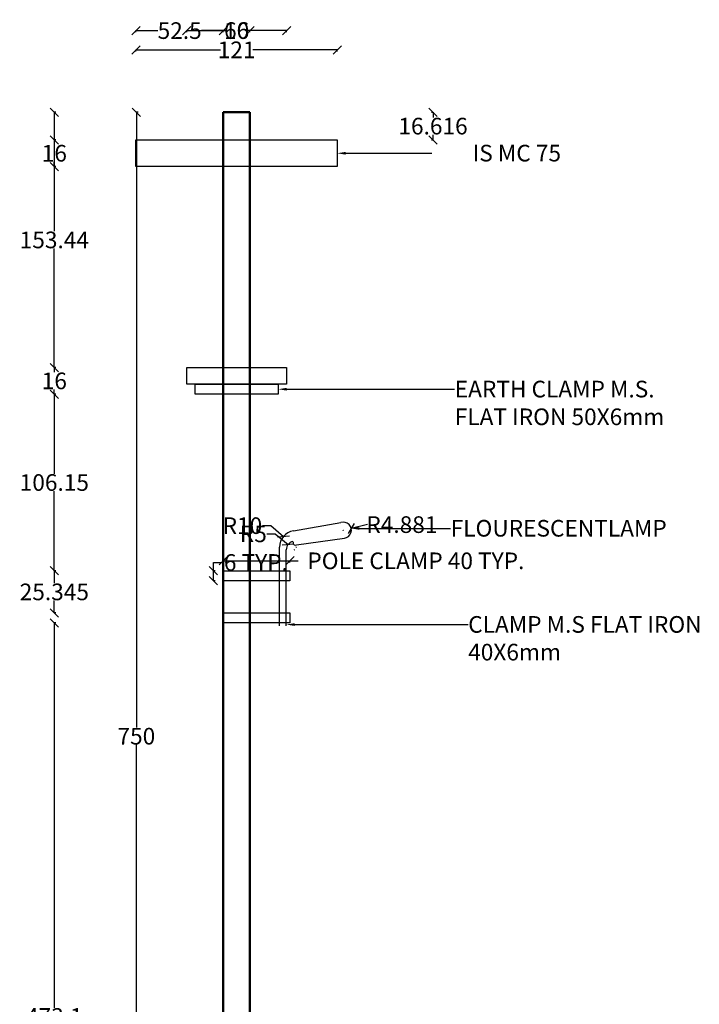
# Model space of a CAD drawing. Units: centimetres. Extents: x -70 to 1009, y -133 to 977.
# Tile 2 of 3: x -70 to 338, y 385 to 977. Entities that reach past the tile are written whole.
import ezdxf
from ezdxf import colors
from ezdxf.entities.mleader import LeaderData, LeaderLine
from ezdxf.math import Vec2, Vec3

# ---------------------------------------------------------------- set-up
doc = ezdxf.new("R2010")
doc.units = ezdxf.units.CM
doc.header["$MEASUREMENT"] = 0
for name, color, linetype, lineweight in [('E-ANNO-DIMS', 2, 'Continuous', 18), ('E-ANNO-TEXT', 7, 'Continuous', 25), ('E-LITE', 3, 'Continuous', 25), ('E-POLE', 7, 'Continuous', 50), ('E-POLE-HDWR', 4, 'Continuous', 25)]:
    doc.layers.add(name, color=color, linetype=linetype, lineweight=lineweight)
doc.styles.get("Standard").update_dxf_attribs({"font": 'arial.ttf'})
doc.dimstyles.get("Standard").update_dxf_attribs({"dimtxt": 10, "dimasz": 5, "dimexe": 0.1, "dimexo": 0.1, "dimgap": 0.09, "dimtad": 0, "dimtih": 1, "dimtoh": 1, "dimdec": 0, "dimzin": 0, "dimdsep": 46, "dimtxsty": 'Standard', "dimblk": 'OBLIQUE', "dimcen": 0.09, "dimadec": 0, "dimazin": 0, "dimtfac": 1, "dimtdec": 0, "dimtofl": 0, "dimtmove": 0, "dimatfit": 3, "dimfxl": 1, "dimfxlon": 1, "dimtolj": 1, "dimtzin": 0, "dimarcsym": 0})

# ---------------------------------------------------------------- blocks, each defined once
blk = doc.blocks.new('_Oblique')
at = {"color": 0, "linetype": 'ByBlock', "lineweight": -2}
blk.add_line((-0.5, -0.5), (0.5, 0.5), dxfattribs=at)
blk = doc.blocks.new('*D1')
at = {"layer": 'Defpoints', "color": 0, "transparency": 16777216}
for p in [(120.74, 958.75), (-0.26, 904.6), (120.74, 904.6)]:
    blk.add_point(p, dxfattribs=at)
at = {"layer": 'E-ANNO-DIMS', "color": 0, "lineweight": -2, "transparency": 16777216}
for p, q in [((-0.26, 957.75), (-0.26, 958.85)), ((-0.26, 958.75), (50.54, 958.75)), ((120.74, 958.75), (69.94, 958.75)), ((120.74, 957.75), (120.74, 958.85))]:
    blk.add_line(p, q, dxfattribs=at)
at = {"layer": 'E-ANNO-DIMS', "color": 0, "lineweight": -2, "transparency": 16777216, "xscale": 5, "yscale": 5, "zscale": 5, "rotation": 180}
blk.add_blockref('_Oblique', (-0.26, 958.75), dxfattribs=at)
at = {"layer": 'E-ANNO-DIMS', "color": 0, "lineweight": -2, "transparency": 16777216, "xscale": 5, "yscale": 5, "zscale": 5}
blk.add_blockref('_Oblique', (120.74, 958.75), dxfattribs=at)
at = {"layer": 'E-ANNO-DIMS', "color": 0, "transparency": 16777216, "insert": (60.24, 958.75), "char_height": 10, "attachment_point": 5}
blk.add_mtext('\\A1;121', dxfattribs=at)
blk = doc.blocks.new('*D3')
at = {"layer": 'Defpoints', "color": 0, "transparency": 16777216}
for p in [(52.24, 921.22), (-0.04, 171.22), (52.24, 171.22)]:
    blk.add_point(p, dxfattribs=at)
at = {"layer": 'E-ANNO-DIMS', "color": 0, "lineweight": -2, "transparency": 16777216}
for p, q in [((0.96, 921.22), (-0.14, 921.22)), ((-0.04, 921.22), (-0.04, 551.41)), ((-0.04, 171.22), (-0.04, 541.02)), ((0.96, 171.22), (-0.14, 171.22))]:
    blk.add_line(p, q, dxfattribs=at)
at = {"layer": 'E-ANNO-DIMS', "color": 0, "lineweight": -2, "transparency": 16777216, "xscale": 5, "yscale": 5, "zscale": 5}
for p, rotation in [((-0.04, 921.22), 90), ((-0.04, 171.22), 270)]:
    blk.add_blockref('_Oblique', p, dxfattribs=dict(at, rotation=rotation))
at = {"layer": 'E-ANNO-DIMS', "color": 0, "transparency": 16777216, "insert": (-0.04, 546.22), "char_height": 10, "attachment_point": 5}
blk.add_mtext('\\A1;750', dxfattribs=at)
blk = doc.blocks.new('POLE-CLAMP')
for p, q in [((0, 0), (0, 6)), ((0, 6), (40, 6)), ((40, 6), (40, 0)), ((40, 0), (0, 0))]:
    blk.add_line(p, q)
blk = doc.blocks.new('*D19')
at = {"layer": 'Defpoints', "color": 0, "transparency": 16777216}
for p in [(92.24, 651.63), (52.24, 645.63), (92.24, 645.63)]:
    blk.add_point(p, dxfattribs=at)
at = {"layer": 'E-ANNO-DIMS', "color": 0, "lineweight": -2, "transparency": 16777216}
for p, q in [((52.24, 650.63), (52.24, 651.73)), ((52.24, 651.63), (92.24, 651.63)), ((92.24, 650.63), (92.24, 651.73)), ((92.24, 651.63), (97.24, 651.63))]:
    blk.add_line(p, q, dxfattribs=at)
at = {"layer": 'E-ANNO-DIMS', "color": 0, "lineweight": -2, "transparency": 16777216, "xscale": 5, "yscale": 5, "zscale": 5, "rotation": 180}
blk.add_blockref('_Oblique', (52.24, 651.63), dxfattribs=at)
at = {"layer": 'E-ANNO-DIMS', "color": 0, "lineweight": -2, "transparency": 16777216, "xscale": 5, "yscale": 5, "zscale": 5}
blk.add_blockref('_Oblique', (92.24, 651.63), dxfattribs=at)
at = {"layer": 'E-ANNO-DIMS', "color": 0, "transparency": 16777216, "insert": (168, 651.63), "char_height": 10, "attachment_point": 5}
blk.add_mtext('\\A1;POLE CLAMP 40 TYP.', dxfattribs=at)
blk = doc.blocks.new('*D20')
at = {"layer": 'Defpoints', "color": 0, "transparency": 16777216}
for p in [(46.24, 645.63), (52.24, 645.63), (52.24, 639.63)]:
    blk.add_point(p, dxfattribs=at)
at = {"layer": 'E-ANNO-DIMS', "color": 0, "lineweight": -2, "transparency": 16777216}
for p, q in [((47.24, 645.63), (46.14, 645.63)), ((46.24, 645.63), (46.24, 650.63)), ((46.24, 650.63), (51.24, 650.63)), ((46.24, 639.63), (46.24, 645.63)), ((47.24, 639.63), (46.14, 639.63))]:
    blk.add_line(p, q, dxfattribs=at)
at = {"layer": 'E-ANNO-DIMS', "color": 0, "lineweight": -2, "transparency": 16777216, "xscale": 5, "yscale": 5, "zscale": 5}
for p, rotation in [((46.24, 645.63), 90), ((46.24, 639.63), 270)]:
    blk.add_blockref('_Oblique', p, dxfattribs=dict(at, rotation=rotation))
at = {"layer": 'E-ANNO-DIMS', "color": 0, "transparency": 16777216, "insert": (71.81, 650.63), "char_height": 10, "attachment_point": 5}
blk.add_mtext('\\A1;6 TYP.', dxfattribs=at)
blk = doc.blocks.new('*D24')
at = {"layer": 'Defpoints', "color": 0, "transparency": 16777216}
for p in [(68.24, 970.32), (52.24, 921.22), (68.24, 921.22)]:
    blk.add_point(p, dxfattribs=at)
at = {"layer": 'E-ANNO-DIMS', "color": 0, "lineweight": -2, "transparency": 16777216}
for p, q in [((52.24, 969.32), (52.24, 970.42)), ((52.24, 970.32), (53.46, 970.32)), ((68.24, 970.32), (67.02, 970.32)), ((68.24, 969.32), (68.24, 970.42))]:
    blk.add_line(p, q, dxfattribs=at)
at = {"layer": 'E-ANNO-DIMS', "color": 0, "lineweight": -2, "transparency": 16777216, "xscale": 5, "yscale": 5, "zscale": 5, "rotation": 180}
blk.add_blockref('_Oblique', (52.24, 970.32), dxfattribs=at)
at = {"layer": 'E-ANNO-DIMS', "color": 0, "lineweight": -2, "transparency": 16777216, "xscale": 5, "yscale": 5, "zscale": 5}
blk.add_blockref('_Oblique', (68.24, 970.32), dxfattribs=at)
at = {"layer": 'E-ANNO-DIMS', "color": 0, "transparency": 16777216, "insert": (60.24, 970.32), "char_height": 10, "attachment_point": 5}
blk.add_mtext('\\A1;16', dxfattribs=at)
blk = doc.blocks.new('*D26')
at = {"layer": 'Defpoints', "color": 0, "transparency": 16777216}
for p in [(68.24, 921.22), (120.74, 904.6), (178.32, 904.6)]:
    blk.add_point(p, dxfattribs=at)
at = {"layer": 'E-ANNO-DIMS', "color": 0, "lineweight": -2, "transparency": 16777216}
for p, q in [((177.32, 921.22), (178.42, 921.22)), ((178.32, 921.22), (178.32, 918.1)), ((178.32, 904.6), (178.32, 907.71)), ((177.32, 904.6), (178.42, 904.6))]:
    blk.add_line(p, q, dxfattribs=at)
at = {"layer": 'E-ANNO-DIMS', "color": 0, "lineweight": -2, "transparency": 16777216, "xscale": 5, "yscale": 5, "zscale": 5}
for p, rotation in [((178.32, 921.22), 90), ((178.32, 904.6), 270)]:
    blk.add_blockref('_Oblique', p, dxfattribs=dict(at, rotation=rotation))
at = {"layer": 'E-ANNO-DIMS', "color": 0, "transparency": 16777216, "insert": (178.32, 912.91), "char_height": 10, "attachment_point": 5}
blk.add_mtext('\\A1;16.616', dxfattribs=at)
blk = doc.blocks.new('*D27')
at = {"layer": 'Defpoints', "color": 0, "transparency": 16777216}
for p in [(-49.36, 904.6), (-0.26, 904.6), (-0.26, 888.6)]:
    blk.add_point(p, dxfattribs=at)
at = {"layer": 'E-ANNO-DIMS', "color": 0, "lineweight": -2, "transparency": 16777216}
for p, q in [((-48.36, 904.6), (-49.46, 904.6)), ((-49.36, 904.6), (-49.36, 901.8)), ((-48.36, 888.6), (-49.46, 888.6)), ((-49.36, 888.6), (-49.36, 891.4))]:
    blk.add_line(p, q, dxfattribs=at)
at = {"layer": 'E-ANNO-DIMS', "color": 0, "lineweight": -2, "transparency": 16777216, "xscale": 5, "yscale": 5, "zscale": 5}
for p, rotation in [((-49.36, 904.6), 90), ((-49.36, 888.6), 270)]:
    blk.add_blockref('_Oblique', p, dxfattribs=dict(at, rotation=rotation))
at = {"layer": 'E-ANNO-DIMS', "color": 0, "transparency": 16777216, "insert": (-49.36, 896.6), "char_height": 10, "attachment_point": 5}
blk.add_mtext('\\A1;16', dxfattribs=at)
blk = doc.blocks.new('*D28')
at = {"layer": 'Defpoints', "color": 0, "transparency": 16777216}
for p in [(52.24, 970.32), (52.24, 921.22), (-0.26, 904.6)]:
    blk.add_point(p, dxfattribs=at)
at = {"layer": 'E-ANNO-DIMS', "color": 0, "lineweight": -2, "transparency": 16777216}
for p, q in [((-0.26, 969.32), (-0.26, 970.42)), ((-0.26, 970.32), (12.87, 970.32)), ((52.24, 970.32), (39.1, 970.32)), ((52.24, 969.32), (52.24, 970.42))]:
    blk.add_line(p, q, dxfattribs=at)
at = {"layer": 'E-ANNO-DIMS', "color": 0, "lineweight": -2, "transparency": 16777216, "xscale": 5, "yscale": 5, "zscale": 5, "rotation": 180}
blk.add_blockref('_Oblique', (-0.26, 970.32), dxfattribs=at)
at = {"layer": 'E-ANNO-DIMS', "color": 0, "lineweight": -2, "transparency": 16777216, "xscale": 5, "yscale": 5, "zscale": 5}
blk.add_blockref('_Oblique', (52.24, 970.32), dxfattribs=at)
at = {"layer": 'E-ANNO-DIMS', "color": 0, "transparency": 16777216, "insert": (25.99, 970.32), "char_height": 10, "attachment_point": 5}
blk.add_mtext('\\A1;52.5', dxfattribs=at)
blk = doc.blocks.new('*D29')
at = {"layer": 'Defpoints', "color": 0, "transparency": 16777216}
for p in [(90.24, 970.32), (30.24, 767.78), (90.24, 767.78)]:
    blk.add_point(p, dxfattribs=at)
at = {"layer": 'E-ANNO-DIMS', "color": 0, "lineweight": -2, "transparency": 16777216}
for p, q in [((30.24, 969.32), (30.24, 970.42)), ((30.24, 970.32), (52.98, 970.32)), ((90.24, 970.32), (67.5, 970.32)), ((90.24, 969.32), (90.24, 970.42))]:
    blk.add_line(p, q, dxfattribs=at)
at = {"layer": 'E-ANNO-DIMS', "color": 0, "lineweight": -2, "transparency": 16777216, "xscale": 5, "yscale": 5, "zscale": 5, "rotation": 180}
blk.add_blockref('_Oblique', (30.24, 970.32), dxfattribs=at)
at = {"layer": 'E-ANNO-DIMS', "color": 0, "lineweight": -2, "transparency": 16777216, "xscale": 5, "yscale": 5, "zscale": 5}
blk.add_blockref('_Oblique', (90.24, 970.32), dxfattribs=at)
at = {"layer": 'E-ANNO-DIMS', "color": 0, "transparency": 16777216, "insert": (60.24, 970.32), "char_height": 10, "attachment_point": 5}
blk.add_mtext('\\A1;60', dxfattribs=at)
blk = doc.blocks.new('*D30')
at = {"layer": 'Defpoints', "color": 0, "transparency": 16777216}
for p in [(30.24, 767.78), (-49.36, 751.78), (35.24, 751.78)]:
    blk.add_point(p, dxfattribs=at)
at = {"layer": 'E-ANNO-DIMS', "color": 0, "lineweight": -2, "transparency": 16777216}
for p, q in [((-48.36, 767.78), (-49.46, 767.78)), ((-49.36, 767.78), (-49.36, 764.97)), ((-48.36, 751.78), (-49.46, 751.78)), ((-49.36, 751.78), (-49.36, 754.58))]:
    blk.add_line(p, q, dxfattribs=at)
at = {"layer": 'E-ANNO-DIMS', "color": 0, "lineweight": -2, "transparency": 16777216, "xscale": 5, "yscale": 5, "zscale": 5}
for p, rotation in [((-49.36, 767.78), 90), ((-49.36, 751.78), 270)]:
    blk.add_blockref('_Oblique', p, dxfattribs=dict(at, rotation=rotation))
at = {"layer": 'E-ANNO-DIMS', "color": 0, "transparency": 16777216, "insert": (-49.36, 759.78), "char_height": 10, "attachment_point": 5}
blk.add_mtext('\\A1;16', dxfattribs=at)
blk = doc.blocks.new('*D31')
at = {"layer": 'Defpoints', "color": 0, "transparency": 16777216}
for p in [(52.24, 921.22), (-49.36, 767.78), (30.24, 767.78)]:
    blk.add_point(p, dxfattribs=at)
at = {"layer": 'E-ANNO-DIMS', "color": 0, "lineweight": -2, "transparency": 16777216}
for p, q in [((-48.36, 921.22), (-49.46, 921.22)), ((-49.36, 921.22), (-49.36, 849.69)), ((-49.36, 767.78), (-49.36, 839.3)), ((-48.36, 767.78), (-49.46, 767.78))]:
    blk.add_line(p, q, dxfattribs=at)
at = {"layer": 'E-ANNO-DIMS', "color": 0, "lineweight": -2, "transparency": 16777216, "xscale": 5, "yscale": 5, "zscale": 5}
for p, rotation in [((-49.36, 921.22), 90), ((-49.36, 767.78), 270)]:
    blk.add_blockref('_Oblique', p, dxfattribs=dict(at, rotation=rotation))
at = {"layer": 'E-ANNO-DIMS', "color": 0, "transparency": 16777216, "insert": (-49.36, 844.5), "char_height": 10, "attachment_point": 5}
blk.add_mtext('\\A1;153.44', dxfattribs=at)
blk = doc.blocks.new('*D32')
at = {"layer": 'Defpoints', "color": 0, "transparency": 16777216}
for p in [(35.24, 751.78), (-49.36, 645.63), (52.24, 645.63)]:
    blk.add_point(p, dxfattribs=at)
at = {"layer": 'E-ANNO-DIMS', "color": 0, "lineweight": -2, "transparency": 16777216}
for p, q in [((-48.36, 751.78), (-49.46, 751.78)), ((-49.36, 751.78), (-49.36, 703.9)), ((-49.36, 645.63), (-49.36, 693.5)), ((-48.36, 645.63), (-49.46, 645.63))]:
    blk.add_line(p, q, dxfattribs=at)
at = {"layer": 'E-ANNO-DIMS', "color": 0, "lineweight": -2, "transparency": 16777216, "xscale": 5, "yscale": 5, "zscale": 5}
for p, rotation in [((-49.36, 751.78), 90), ((-49.36, 645.63), 270)]:
    blk.add_blockref('_Oblique', p, dxfattribs=dict(at, rotation=rotation))
at = {"layer": 'E-ANNO-DIMS', "color": 0, "transparency": 16777216, "insert": (-49.36, 698.7), "char_height": 10, "attachment_point": 5}
blk.add_mtext('\\A1;106.15', dxfattribs=at)
blk = doc.blocks.new('*D33')
at = {"layer": 'Defpoints', "color": 0, "transparency": 16777216}
for p in [(52.24, 645.63), (-49.36, 620.28), (52.24, 620.28)]:
    blk.add_point(p, dxfattribs=at)
at = {"layer": 'E-ANNO-DIMS', "color": 0, "lineweight": -2, "transparency": 16777216}
for p, q in [((-48.36, 645.63), (-49.46, 645.63)), ((-49.36, 645.63), (-49.36, 638.15)), ((-49.36, 620.28), (-49.36, 627.75)), ((-48.36, 620.28), (-49.46, 620.28))]:
    blk.add_line(p, q, dxfattribs=at)
at = {"layer": 'E-ANNO-DIMS', "color": 0, "lineweight": -2, "transparency": 16777216, "xscale": 5, "yscale": 5, "zscale": 5}
for p, rotation in [((-49.36, 645.63), 90), ((-49.36, 620.28), 270)]:
    blk.add_blockref('_Oblique', p, dxfattribs=dict(at, rotation=rotation))
at = {"layer": 'E-ANNO-DIMS', "color": 0, "transparency": 16777216, "insert": (-49.36, 632.95), "char_height": 10, "attachment_point": 5}
blk.add_mtext('\\A1;25.345', dxfattribs=at)
blk = doc.blocks.new('*D34')
at = {"layer": 'Defpoints', "color": 0, "transparency": 16777216}
for p in [(52.24, 614.28), (-49.36, 141.22), (2.39, 141.22)]:
    blk.add_point(p, dxfattribs=at)
at = {"layer": 'E-ANNO-DIMS', "color": 0, "lineweight": -2, "transparency": 16777216}
for p, q in [((-48.36, 614.28), (-49.46, 614.28)), ((-49.36, 614.28), (-49.36, 382.95)), ((-49.36, 141.22), (-49.36, 372.55)), ((-48.36, 141.22), (-49.46, 141.22))]:
    blk.add_line(p, q, dxfattribs=at)
at = {"layer": 'E-ANNO-DIMS', "color": 0, "lineweight": -2, "transparency": 16777216, "xscale": 5, "yscale": 5, "zscale": 5}
for p, rotation in [((-49.36, 614.28), 90), ((-49.36, 141.22), 270)]:
    blk.add_blockref('_Oblique', p, dxfattribs=dict(at, rotation=rotation))
at = {"layer": 'E-ANNO-DIMS', "color": 0, "transparency": 16777216, "insert": (-49.36, 377.75), "char_height": 10, "attachment_point": 5}
blk.add_mtext('\\A1;473.1', dxfattribs=at)
blk = doc.blocks.new('*D35')
at = {"layer": 'Defpoints', "color": 0, "transparency": 16777216}
for p in [(52.23894, 639.625874), (86.058746, 612.513226), (86.058746, -27.884542)]:
    blk.add_point(p, dxfattribs=at)
at = {"layer": 'E-ANNO-DIMS', "color": 0, "lineweight": -2, "transparency": 16777216}
for p, q in [((52.23894, -27.884542), (47.23894, -27.884542)), ((52.23894, -26.884542), (52.23894, -27.984542)), ((86.058746, -26.884542), (86.058746, -27.984542)), ((86.058746, -27.884542), (91.058746, -27.884542))]:
    blk.add_line(p, q, dxfattribs=at)
at = {"layer": 'E-ANNO-DIMS', "color": 0, "lineweight": -2, "transparency": 16777216, "xscale": 5, "yscale": 5, "zscale": 5}
blk.add_blockref('_Oblique', (52.23894, -27.884542), dxfattribs=at)
at = {"layer": 'E-ANNO-DIMS', "color": 0, "lineweight": -2, "transparency": 16777216, "xscale": 5, "yscale": 5, "zscale": 5, "rotation": 180}
blk.add_blockref('_Oblique', (86.058746, -27.884542), dxfattribs=at)
at = {"layer": 'E-ANNO-DIMS', "color": 0, "transparency": 16777216, "insert": (69.148843, -27.884542), "char_height": 10, "attachment_point": 5}
blk.add_mtext('\\A1;33.82', dxfattribs=at)
blk = doc.blocks.new('*D36')
at = {"layer": 'Defpoints', "color": 0, "transparency": 16777216}
for p in [(129.1, 671.11), (86.06, 612.51), (129.1, -27.88)]:
    blk.add_point(p, dxfattribs=at)
at = {"layer": 'E-ANNO-DIMS', "color": 0, "lineweight": -2, "transparency": 16777216}
for p, q in [((86.06, -26.88), (86.06, -27.98)), ((86.06, -27.88), (90.43, -27.88)), ((129.1, -27.88), (124.72, -27.88)), ((129.1, -26.88), (129.1, -27.98))]:
    blk.add_line(p, q, dxfattribs=at)
at = {"layer": 'E-ANNO-DIMS', "color": 0, "lineweight": -2, "transparency": 16777216, "xscale": 5, "yscale": 5, "zscale": 5, "rotation": 180}
blk.add_blockref('_Oblique', (86.06, -27.88), dxfattribs=at)
at = {"layer": 'E-ANNO-DIMS', "color": 0, "lineweight": -2, "transparency": 16777216, "xscale": 5, "yscale": 5, "zscale": 5}
blk.add_blockref('_Oblique', (129.1, -27.88), dxfattribs=at)
at = {"layer": 'E-ANNO-DIMS', "color": 0, "transparency": 16777216, "insert": (107.58, -27.88), "char_height": 10, "attachment_point": 5}
blk.add_mtext('\\A1;43.04', dxfattribs=at)
blk = doc.blocks.new('*D50')
at = {"layer": 'Defpoints', "color": 0, "transparency": 16777216}
for p in [(88.41, 666.32), (96.06, 659.88)]:
    blk.add_point(p, dxfattribs=at)
at = {"layer": 'E-ANNO-DIMS', "color": 0, "lineweight": -2, "transparency": 16777216}
for p, q in [((75.76, 672.76), (80.76, 672.76)), ((80.76, 672.76), (88.41, 666.32)), ((95.97, 659.88), (96.15, 659.88)), ((96.06, 659.79), (96.06, 659.97))]:
    blk.add_line(p, q, dxfattribs=at)
at = {"layer": 'E-ANNO-DIMS', "color": 0, "lineweight": -2, "transparency": 16777216, "xscale": 5, "yscale": 5, "zscale": 5, "rotation": 319.8963376320703}
blk.add_blockref('_Oblique', (88.41, 666.32), dxfattribs=at)
at = {"layer": 'E-ANNO-DIMS', "color": 0, "transparency": 16777216, "insert": (63.74, 672.76), "char_height": 10, "attachment_point": 5}
blk.add_mtext('\\A1;R10', dxfattribs=at)
blk = doc.blocks.new('*D51')
at = {"layer": 'Defpoints', "color": 0, "transparency": 16777216}
for p in [(91.2, 661.49), (95.06, 658.31)]:
    blk.add_point(p, dxfattribs=at)
at = {"layer": 'E-ANNO-DIMS', "color": 0, "lineweight": -2, "transparency": 16777216}
for p, q in [((78.48, 667.85), (83.48, 667.85)), ((83.48, 667.85), (91.2, 661.49)), ((94.97, 658.31), (95.15, 658.31)), ((95.06, 658.22), (95.06, 658.4))]:
    blk.add_line(p, q, dxfattribs=at)
at = {"layer": 'E-ANNO-DIMS', "color": 0, "lineweight": -2, "transparency": 16777216, "xscale": 5, "yscale": 5, "zscale": 5, "rotation": 320.5311387777274}
blk.add_blockref('_Oblique', (91.2, 661.49), dxfattribs=at)
at = {"layer": 'E-ANNO-DIMS', "color": 0, "transparency": 16777216, "insert": (70.29, 667.85), "char_height": 10, "attachment_point": 5}
blk.add_mtext('\\A1;R5', dxfattribs=at)
blk = doc.blocks.new('*D52')
at = {"layer": 'Defpoints', "color": 0, "transparency": 16777216}
for p in [(124.34, 670), (129.1, 671.11)]:
    blk.add_point(p, dxfattribs=at)
at = {"layer": 'E-ANNO-DIMS', "color": 0, "lineweight": -2, "transparency": 16777216}
for p, q in [((124.25, 670), (124.43, 670)), ((124.34, 669.91), (124.34, 670.09)), ((138.83, 673.4), (129.1, 671.11))]:
    blk.add_line(p, q, dxfattribs=at)
at = {"layer": 'E-ANNO-DIMS', "color": 0, "lineweight": -2, "transparency": 16777216, "xscale": 5, "yscale": 5, "zscale": 5, "rotation": 193.2029927353141}
blk.add_blockref('_Oblique', (129.1, 671.11), dxfattribs=at)
at = {"layer": 'E-ANNO-DIMS', "color": 0, "transparency": 16777216, "insert": (159.61, 673.4), "char_height": 10, "attachment_point": 5}
blk.add_mtext('\\A1;R4.881', dxfattribs=at)

msp = doc.modelspace()

# ---------------------------------------------------------------- linework, layer by layer
at = {"layer": 'E-LITE'}
for p, q in [((94.3576, 669.7296), (122.8867, 674.6545)), ((96.1413, 661.139), (125.11, 665.1762)), ((86.0587, 612.5132), (86.0587, 659.8753)), ((90.0587, 612.5132), (90.0587, 658.3118))]:
    msp.add_line(p, q, dxfattribs=at)
for centre, radius, start, end in [((124.3435, 669.9963), 4.8807, 279.0354675, 107.3674163), ((96.0587, 659.8753), 10, 99.7942626, 180), ((95.0587, 658.3118), 5, 101.0515884, 180)]:
    msp.add_arc(centre, radius, start, end, dxfattribs=at)
msp.add_open_spline([(94.1003, 663.2191), (94.2148, 662.3029), (94.3928, 660.8775), (95.6811, 661.0702), (96.1413, 661.139)], degree=3, knots=[0, 0, 0, 0, 2.22934739, 3.46823679, 3.46823679, 3.46823679, 3.46823679], dxfattribs=at)
at = {"layer": 'E-POLE'}
for p, q in [((52.2389, 171.2155), (52.2389, 921.2155)), ((52.2389, 921.2155), (68.2389, 921.2155)), ((68.2389, 171.2155), (68.2389, 921.2155))]:
    msp.add_line(p, q, dxfattribs=at)
at = {"layer": 'E-POLE-HDWR'}
for p, q in [((-0.2611, 888.5994), (-0.2611, 904.5994)), ((-0.2611, 904.5994), (120.7389, 904.5994)), ((120.7389, 904.5994), (120.7389, 888.5994)), ((120.7389, 888.5994), (-0.2611, 888.5994)), ((30.2389, 757.7753), (30.2389, 767.7753)), ((30.2389, 767.7753), (90.2389, 767.7753)), ((90.2389, 767.7753), (90.2389, 757.7753)), ((90.2389, 757.7753), (30.2389, 757.7753)), ((35.2389, 757.7753), (85.2389, 757.7753)), ((35.2389, 751.7753), (35.2389, 757.7753)), ((85.2389, 757.7753), (85.2389, 751.7753)), ((85.2389, 751.7753), (35.2389, 751.7753))]:
    msp.add_line(p, q, dxfattribs=at)

# ---------------------------------------------------------------- block references
for p in [(52.239, 639.626), (52.239, 614.281)]:
    msp.add_blockref('POLE-CLAMP', p, dxfattribs=at)

# ---------------------------------------------------------------- dimensions: what is measured, and where the dimension line sits
at = {"layer": 'E-ANNO-DIMS'}
for base, p1, p2, override, picture, middle in [((52.2389, 970.3155), (-0.2611, 904.5994), (52.2389, 921.2155), {"dimdec": 1, "dimlfac": 1, "dimrnd": 0, "dimzin": 0, "dimdsep": 46, "dimlunit": 2}, '*D28', (25.9889, 970.3155)), ((90.2389, 970.3155), (30.2389, 767.7753), (90.2389, 767.7753), {"dimdec": 0, "dimlfac": 1, "dimrnd": 0, "dimzin": 0, "dimdsep": 46, "dimlunit": 2}, '*D29', (60.2389, 970.3155)), ((68.2389, 970.3155), (52.2389, 921.2155), (68.2389, 921.2155), {"dimdec": 0, "dimlfac": 1, "dimrnd": 0, "dimzin": 0, "dimdsep": 46, "dimlunit": 2}, '*D24', (60.2389, 970.3155)), ((120.7389, 958.7524), (-0.2611, 904.5994), (120.7389, 904.5994), {"dimclrd": 0, "dimclre": 0, "dimclrt": 0}, '*D1', (60.2389, 958.7524)), ((129.0952, -27.8845), (86.0587, 612.5132), (129.0952, 671.1109), {"dimdec": 2, "dimlfac": 1, "dimrnd": 0, "dimzin": 0, "dimdsep": 46, "dimlunit": 2}, '*D36', (107.577, -27.8845)), ((86.0587, -27.8845), (52.2389, 639.6259), (86.0587, 612.5132), {"dimdec": 2, "dimlfac": 1, "dimrnd": 0, "dimzin": 0, "dimdsep": 46, "dimlunit": 2}, '*D35', (69.1488, -27.8845))]:
    dim = msp.add_linear_dim(base=base, p1=p1, p2=p2, dimstyle='Standard', override=override, dxfattribs=at)
    dim.commit()
    dim.dimension.update_dxf_attribs({"geometry": picture, "text_midpoint": middle})
for base, p1, p2, override, picture, middle in [((-49.3611, 767.7753), (52.2389, 921.2155), (30.2389, 767.7753), {"dimdec": 2, "dimlfac": 1, "dimrnd": 0, "dimzin": 0, "dimdsep": 46, "dimlunit": 2}, '*D31', (-49.3611, 844.4954)), ((-0.0426, 171.2155), (52.2389, 921.2155), (52.2389, 171.2155), {"dimclrd": 0, "dimclre": 0, "dimclrt": 0}, '*D3', (-0.0426, 546.2155)), ((178.3203, 904.5994), (68.2389, 921.2155), (120.7389, 904.5994), {"dimdec": 3, "dimlfac": 1, "dimrnd": 0, "dimzin": 0, "dimdsep": 46, "dimlunit": 2}, '*D26', (178.3203, 912.9074)), ((-49.3611, 904.5994), (-0.2611, 888.5994), (-0.2611, 904.5994), {"dimdec": 0, "dimlfac": 1, "dimrnd": 0, "dimzin": 0, "dimdsep": 46, "dimlunit": 2}, '*D27', (-49.3611, 896.5994)), ((-49.3611, 751.7753), (30.2389, 767.7753), (35.2389, 751.7753), {"dimdec": 0, "dimlfac": 1, "dimrnd": 0, "dimzin": 0, "dimdsep": 46, "dimlunit": 2}, '*D30', (-49.3611, 759.7753)), ((-49.3611, 645.6259), (35.2389, 751.7753), (52.2389, 645.6259), {"dimdec": 2, "dimlfac": 1, "dimrnd": 0, "dimzin": 0, "dimdsep": 46, "dimlunit": 2}, '*D32', (-49.3611, 698.7006)), ((-49.3611, 620.2808), (52.2389, 645.6259), (52.2389, 620.2808), {"dimdec": 3, "dimlfac": 1, "dimrnd": 0, "dimzin": 0, "dimdsep": 46, "dimlunit": 2}, '*D33', (-49.3611, 632.9534)), ((-49.3611, 141.2155), (52.2389, 614.2808), (2.3883, 141.2155), {"dimdec": 1, "dimlfac": 1, "dimrnd": 0, "dimzin": 0, "dimdsep": 46, "dimlunit": 2}, '*D34', (-49.3611, 377.7481))]:
    dim = msp.add_linear_dim(base=base, p1=p1, p2=p2, angle=90, dimstyle='Standard', override=override, dxfattribs=at)
    dim.commit()
    dim.dimension.update_dxf_attribs({"geometry": picture, "text_midpoint": middle})
dim = msp.add_linear_dim(base=(92.2389, 651.6259), p1=(52.2389, 645.6259), p2=(92.2389, 645.6259), text='POLE CLAMP <> TYP.', dimstyle='Standard', override={"dimdec": 0, "dimrnd": 0, "dimzin": 0, "dimlunit": 2}, dxfattribs=at)
dim.commit()
dim.dimension.update_dxf_attribs({"geometry": '*D19', "text_midpoint": (168.0008, 651.6259)})
for center, mpoint, override, picture, middle in [((96.0587, 659.8753), (88.4099, 666.317), {"dimdec": 0, "dimlfac": 1, "dimrnd": 0, "dimzin": 0, "dimdsep": 46, "dimlunit": 2}, '*D50', (63.7407, 672.7588)), ((124.3435, 669.9963), (129.0952, 671.111), {"dimdec": 3, "dimlfac": 1, "dimrnd": 0, "dimzin": 0, "dimdsep": 46, "dimlunit": 2}, '*D52', (159.6132, 673.3951)), ((95.0587, 658.3118), (91.1989, 661.4901), {"dimdec": 0, "dimlfac": 1, "dimrnd": 0, "dimzin": 0, "dimdsep": 46, "dimlunit": 2}, '*D51', (70.2889, 667.8467))]:
    dim = msp.add_radius_dim(center=center, mpoint=mpoint, dimstyle='Standard', override=override, dxfattribs=at)
    dim.commit()
    dim.dimension.update_dxf_attribs({"geometry": picture, "text_midpoint": middle})
dim = msp.add_linear_dim(base=(46.2389, 645.6259), p1=(52.2389, 639.6259), p2=(52.2389, 645.6259), angle=90, text='<> TYP.', dimstyle='Standard', override={"dimdec": 0, "dimrnd": 0, "dimzin": 0, "dimlunit": 2}, dxfattribs=at)
dim.commit()
dim.dimension.update_dxf_attribs({"geometry": '*D20', "text_midpoint": (71.8098, 650.6259)})

# ---------------------------------------------------------------- leaders
at = {"layer": 'E-ANNO-TEXT'}
ml = msp.add_multileader_mtext('Standard', dxfattribs=at)
ml.set_content('^IIS MC 75', color=256)
ml.set_leader_properties()
ml.build(insert=Vec2(0, 0))
ml.multileader.update_dxf_attribs({"dogleg_length": 0.36, "arrow_head_size": 5})
ctx = ml.context
ctx.base_point, ctx.char_height, ctx.arrow_head_size, ctx.landing_gap_size, ctx.plane_origin = Vec3(177.585, 896.5994), 10, 5, 0.09, Vec3(120.7389, 896.5994)
notes = []
notes.append((ctx, [(0, (1, 1, 0), (177.225, 896.5994), (1, 0), 0.36, [(0, [(120.7389, 896.5994)], 0, [])])]))
ctx.mtext.insert, ctx.mtext.flow_direction = Vec3(177.675, 901.6846), 5
ml = msp.add_multileader_mtext('Standard', dxfattribs=at)
ml.set_content('EARTH CLAMP M.S.\\PFLAT IRON 50X6mm', color=256)
ml.set_leader_properties()
ml.build(insert=Vec2(0, 0))
ml.multileader.update_dxf_attribs({"dogleg_length": 0.36, "arrow_head_size": 5})
ctx = ml.context
ctx.base_point, ctx.char_height, ctx.arrow_head_size, ctx.landing_gap_size, ctx.plane_origin = Vec3(191.3043, 754.7753), 10, 5, 0.09, Vec3(85.2389, 754.7753)
notes.append((ctx, [(0, (1, 1, 0), (190.9443, 754.7753), (1, 0), 0.36, [(0, [(85.2389, 754.7753)], 0, [])])]))
ctx.mtext.insert, ctx.mtext.flow_direction = Vec3(191.3943, 759.8606), 5
ml = msp.add_multileader_mtext('Standard', dxfattribs=at)
ml.set_content('FLOURESCENTLAMP', color=256)
ml.set_leader_properties()
ml.build(insert=Vec2(0, 0))
ml.multileader.update_dxf_attribs({"dogleg_length": 0.36, "arrow_head_size": 5})
ctx = ml.context
ctx.base_point, ctx.char_height, ctx.arrow_head_size, ctx.landing_gap_size, ctx.plane_origin = Vec3(188.8324, 671.1109), 10, 5, 0.09, Vec3(129.0952, 671.1109)
notes.append((ctx, [(0, (1, 1, 0), (188.4724, 671.1109), (1, 0), 0.36, [(0, [(129.0952, 671.1109)], 0, [])])]))
ctx.mtext.insert, ctx.mtext.flow_direction = Vec3(188.9224, 676.1962), 5
ml = msp.add_multileader_mtext('Standard', dxfattribs=at)
ml.set_content('CLAMP M.S FLAT IRON\\P40X6mm', color=256)
ml.set_leader_properties()
ml.build(insert=Vec2(0, 0))
ml.multileader.update_dxf_attribs({"dogleg_length": 0.36, "arrow_head_size": 5})
ctx = ml.context
ctx.base_point, ctx.char_height, ctx.arrow_head_size, ctx.landing_gap_size, ctx.plane_origin = Vec3(199.3629, 613.3187), 10, 5, 0.09, Vec3(90.0587, 613.3187)
notes.append((ctx, [(0, (1, 1, 0), (199.0029, 613.3187), (1, 0), 0.36, [(0, [(90.0587, 613.3187)], 0, [])])]))
ctx.mtext.insert, ctx.mtext.flow_direction = Vec3(199.4529, 618.4039), 5
for ctx, leaders in notes:
    for number, flags, end, landing, length, lines in leaders:
        leader = LeaderData()
        leader.index, (leader.has_last_leader_line, leader.has_dogleg_vector, leader.attachment_direction) = number, flags
        leader.last_leader_point, leader.dogleg_vector, leader.dogleg_length = Vec3(end), Vec3(landing), length
        for number, points, colour, breaks in lines:
            line = LeaderLine()
            line.index, line.vertices, line.color, line.breaks = number, Vec3.list(points), colors.encode_raw_color(colour), breaks
            leader.lines.append(line)
        ctx.leaders.append(leader)

doc.saveas('drawing.dxf')
